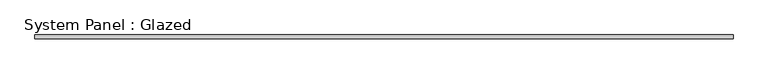
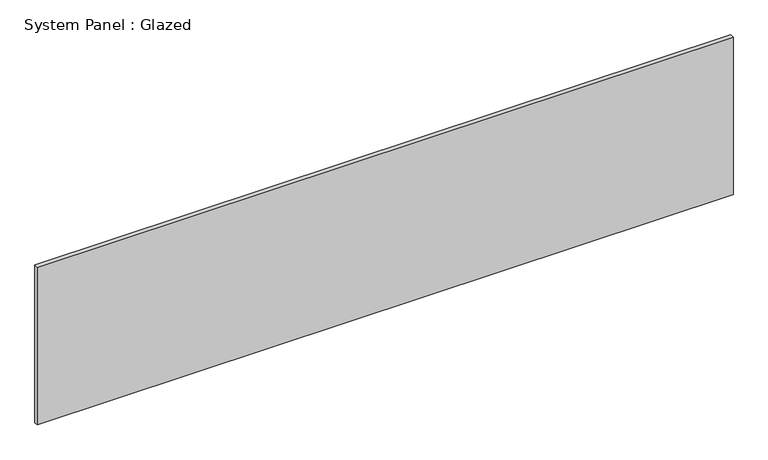
"""IFC4 building model written with IfcOpenShell, lengths in millimetres: plate geometry, System Panel : Glazed."""

from ifc_helpers import new_model, si_unit, origin, origin_with_axes, place, context, project, spatial, polyline, outline, extrude, source, transform, mapped, element, save


def system_panel_glazed_fe37cdeb(model_context):
    return source(origin(), model_context, "Body", "SweptSolid", [
        extrude(outline(polyline([(2410.8509256, 19.05), (-2410.8509256, 19.05), (-2410.8509256, 44.45), (2410.8509256, 44.45), (2410.8509256, 19.05)])), origin_with_axes(), (0.0, 0.0, 1.0), 1155.7),
    ])


if __name__ == "__main__":
    model = new_model("IFC4")
    model_context = context("Model", 3, world=origin())
    ifc_project = project(units=[si_unit("LENGTHUNIT", "METRE", prefix="MILLI")], contexts=[model_context])
    site = spatial("IfcSite", under=ifc_project)
    building = spatial("IfcBuilding", under=site)
    placement = place(None, origin())
    system_panel_glazed_shape = system_panel_glazed_fe37cdeb(model_context)
    element("IfcPlate", 1, ObjectType="System Panel : Glazed", at=placement, inside=building, context=model_context, shape_type="MappedRepresentation", body=[
        mapped(system_panel_glazed_shape, transform((0.0, 0.0, 0.0), x_axis=(1.0, 0.0, 0.0), y_axis=(0.0, 1.0, 0.0), z_axis=(0.0, 0.0, 1.0))),
    ])
    save(model, "model.ifc")

# Revit data of these elements
# Type "System Panel : Glazed"
#   Construction Type Id = "GSP4R"
#   Analytic Construction = "1/8 in Pilkington single glazing"
#   Visual Light Transmittance = 0.9
#   Solar Heat Gain Coefficient = 0.86
#   Heat Transfer Coefficient (U) = 1.18115 BTU/(h·ft²·°F)
# Element 1 (IfcPlate, "System Panel : Glazed")
#   Materials on its faces: "Glass"
# Materials
#   "Glass": class "Glass", colour RGB 0 128 192, transparency 0.75, Description = "Soda Lime Glass", Cost = 0
